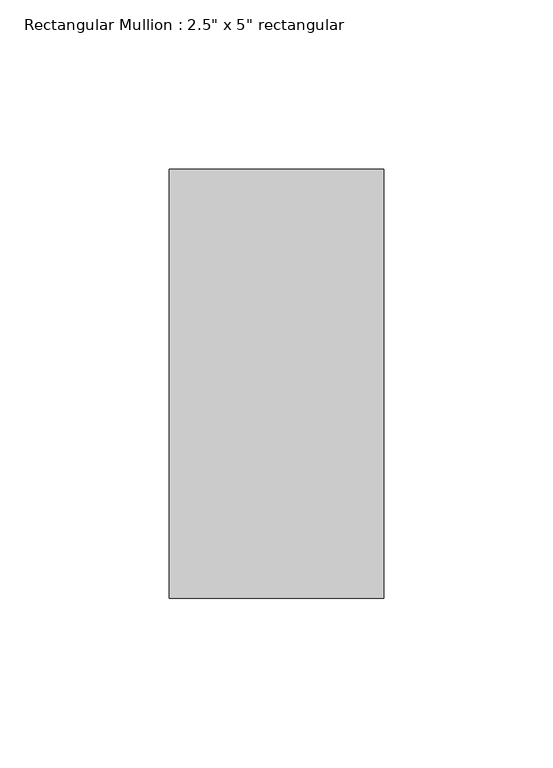
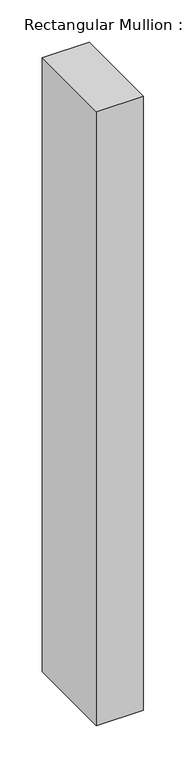
"""IFC4 building model written with IfcOpenShell, lengths in millimetres: member geometry."""

from ifc_helpers import new_model, si_unit, frame, origin, place, context, project, spatial, polyline, outline, extrude, source, transform, mapped, element, save


def member_049a2e78(model_context):
    return source(origin(), model_context, "Body", "SweptSolid", [
        extrude(outline(polyline([(31.75, 63.5), (31.75, -63.5), (-31.75, -63.5), (-31.75, 63.5), (31.75, 63.5)])), frame((0.0, 0.0, -882.65), z_axis=(0.0, 0.0, 1.0), x_axis=(1.0, 0.0, 0.0)), (0.0, 0.0, 1.0), 882.65),
    ])


if __name__ == "__main__":
    model = new_model("IFC4")
    model_context = context("Model", 3, world=origin())
    ifc_project = project(units=[si_unit("LENGTHUNIT", "METRE", prefix="MILLI")], contexts=[model_context])
    site = spatial("IfcSite", under=ifc_project)
    building = spatial("IfcBuilding", under=site)
    placement = place(None, origin())
    member_shape = member_049a2e78(model_context)
    element("IfcMember", 1, ObjectType="Rectangular Mullion : 2.5\" x 5\" rectangular", at=placement, inside=building, context=model_context, shape_type="MappedRepresentation", body=[
        mapped(member_shape, transform((0.0, 0.0, 0.0), x_axis=(1.0, 0.0, 0.0), y_axis=(0.0, 1.0, 0.0), z_axis=(0.0, 0.0, 1.0))),
    ])
    save(model, "model.ifc")

# Revit data of these elements
# Type "Rectangular Mullion : 2.5\" x 5\" rectangular"
#   built-in parameter 1007304 = 0.416667 (stored number, unit not read)
#   built-in parameter 1007301 = 0.104167 (stored number, unit not read)
#   built-in parameter 1007300 = 0.104167 (stored number, unit not read)
# Element 1 (IfcMember, "Rectangular Mullion : 2.5\" x 5\" rectangular")
#   Materials on its faces: "Aluminum"
# Materials
#   "Aluminum": class "Metal", colour RGB 247 247 247, transparency 0, Description = "Aluminum 6061", Cost = 0
